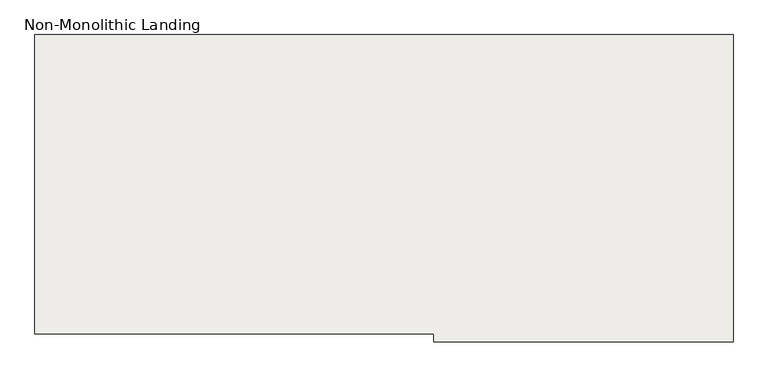
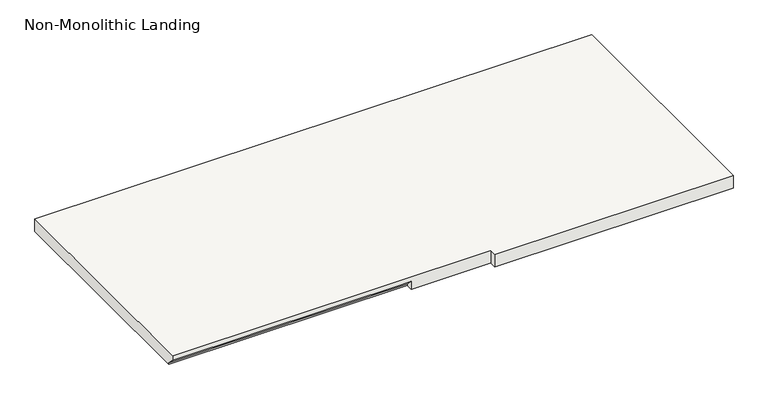
"""IFC4 building model written with IfcOpenShell, lengths in millimetres: slab geometry, Non-Monolithic Landing."""

from ifc_helpers import new_model, si_unit, origin, place, context, project, spatial, faceted_brep, source, transform, mapped, element, save


def non_monolithic_landing_351a0d85(model_context):
    return source(origin(), model_context, "Body", "Brep", [
        faceted_brep([(-3617.4415084, 23194.7216096, 27416.9005799), (-3617.4415084, 23220.1216096, 27391.5005799), (-2703.0415084, 23220.1216096, 27391.5005799), (-2703.0415084, 23194.7216096, 27416.9005799), (-2398.2415084, 23194.7216096, 27435.9505799), (-2398.2415084, 23169.3216096, 27435.9505799), (-1483.8415084, 23169.3216096, 27435.9505799), (-1483.8415084, 23194.7216096, 27435.9505799), (-1483.8415084, 24109.1216096, 27435.9505799), (-3617.4415084, 24109.1216096, 27435.9505799), (-3617.4415084, 23194.7216096, 27435.9505799), (-2703.0415084, 23220.1216096, 27385.1505799), (-3617.4415084, 23220.1216096, 27385.1505799), (-3617.4415084, 24109.1216096, 27385.1505799), (-1483.8415084, 24109.1216096, 27385.1505799), (-1483.8415084, 23194.7216096, 27385.1505799), (-1483.8415084, 23169.3216096, 27385.1505799), (-2398.2415084, 23169.3216096, 27385.1505799), (-2398.2415084, 23194.7216096, 27385.1505799), (-2703.0415084, 23194.7216096, 27385.1505799)], [[[0, 1, 2, 3]], [[4, 5, 6, 7, 8, 9, 10]], [[11, 12, 13, 14, 15, 16, 17, 18, 19]], [[12, 11, 2, 1]], [[11, 19, 3, 2]], [[4, 10, 0, 3, 19, 18]], [[5, 4, 18, 17]], [[6, 5, 17, 16]], [[7, 6, 16, 15]], [[8, 7, 15, 14]], [[9, 8, 14, 13]], [[10, 9, 13, 12, 1, 0]]]),
    ])


if __name__ == "__main__":
    model = new_model("IFC4")
    model_context = context("Model", 3, world=origin())
    ifc_project = project(units=[si_unit("LENGTHUNIT", "METRE", prefix="MILLI")], contexts=[model_context])
    site = spatial("IfcSite", under=ifc_project)
    building = spatial("IfcBuilding", under=site)
    placement = place(None, origin())
    non_monolithic_landing_shape = non_monolithic_landing_351a0d85(model_context)
    element("IfcSlab", 1, ObjectType="Non-Monolithic Landing", at=placement, inside=building, context=model_context, shape_type="MappedRepresentation", body=[
        mapped(non_monolithic_landing_shape, transform((0.0, 0.0, 0.0), x_axis=(1.0, 0.0, 0.0), y_axis=(0.0, 1.0, 0.0), z_axis=(0.0, 0.0, 1.0))),
    ])
    save(model, "model.ifc")
